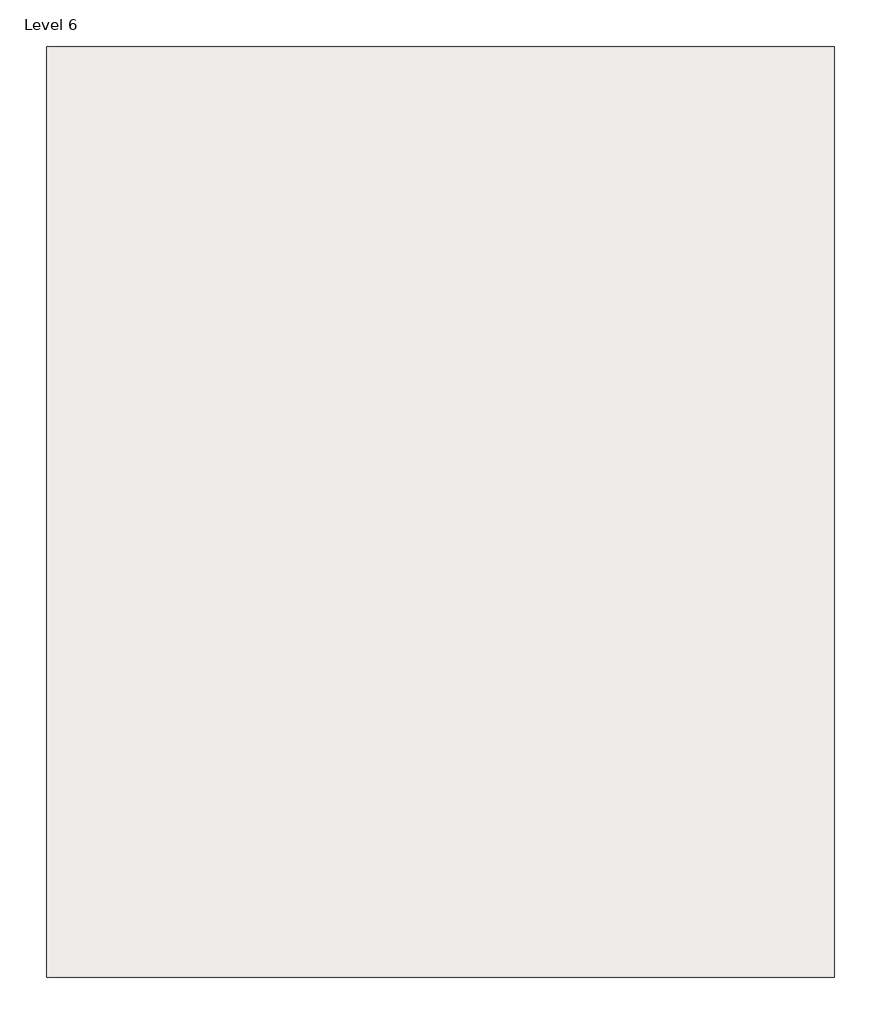
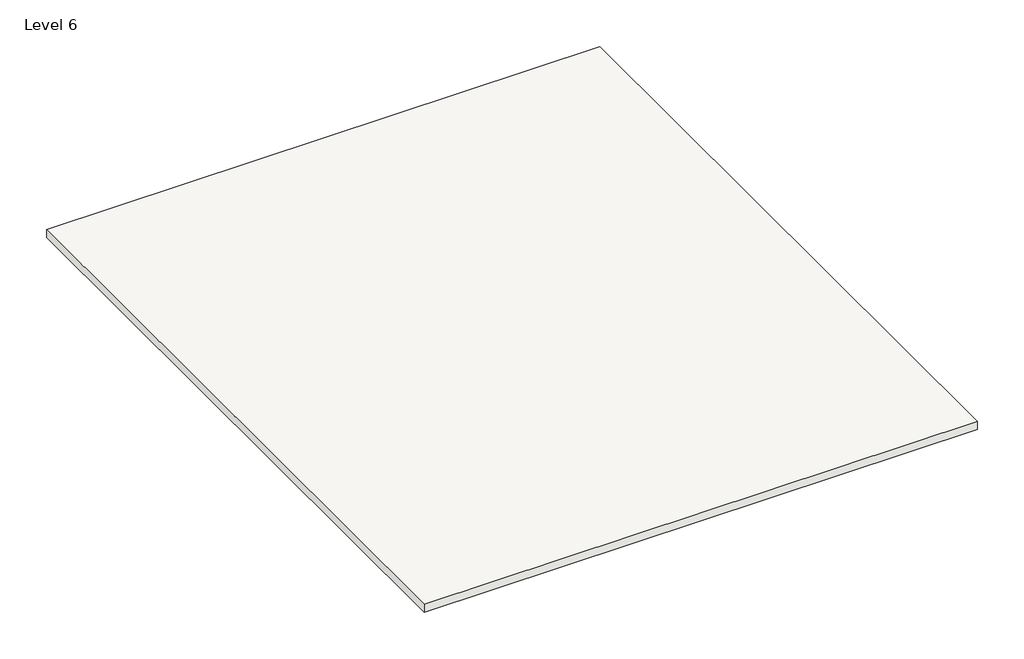
# One storey, incomplete: 1 roof.
"""IFC4 building model written with IfcOpenShell, lengths in millimetres."""

from ifc_helpers import new_model, si_unit, frame, origin, place, context, project, spatial, polyline, outline, extrude, element, save

model = new_model("IFC4")

# Units and contexts
model_context = context("Model", 3, world=origin())
ifc_project = project(units=[si_unit("LENGTHUNIT", "METRE", prefix="MILLI")], contexts=[model_context])

# Site, building, storey
site = spatial("IfcSite", under=ifc_project)
building = spatial("IfcBuilding", under=site)
storey = spatial("IfcBuildingStorey", under=building, Name="Level 6", Elevation=15240.0)

# Roof
placement = place(None, origin())
element("IfcRoof", 1, ObjectType="Generic - 12\"", at=placement, inside=storey, context=model_context, shape_type="SweptSolid", body=[
    extrude(outline(polyline([(2298.7, 13500.1), (12357.1, 13500.1), (12357.1, 1612.9), (2298.7, 1612.9), (2298.7, 13500.1)])), frame((0.0, 0.0, 15240.0), z_axis=(0.0, 0.0, 1.0), x_axis=(1.0, 0.0, 0.0)), (0.0, 0.0, 1.0), 152.4),
])

save(model, "model.ifc")

# Revit data of these elements
# Type "Generic - 12\""
#   Assembly Code = "B1020"
#   Layers, outside or top first: 0' - 6" no material (function 1)
# Element 1 (IfcRoof, "Generic - 12\"")
#   built-in parameter 1001705 = 50.5 (stored number, unit not read)
#   built-in parameter 1001710 = 33615
#   Phase Created = New Construction
#   Materials on its faces: "Clad - White", "Default Roof"
# Materials
#   "Clad - White": class "Wood", colour RGB 242 242 238, transparency 0, Cost = 0
#   "Default Roof": colour RGB 88 101 114, transparency 0, Cost = 0
